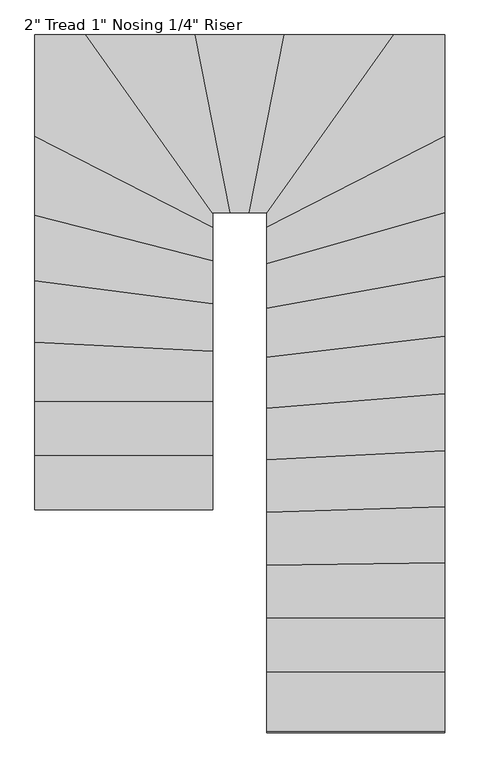
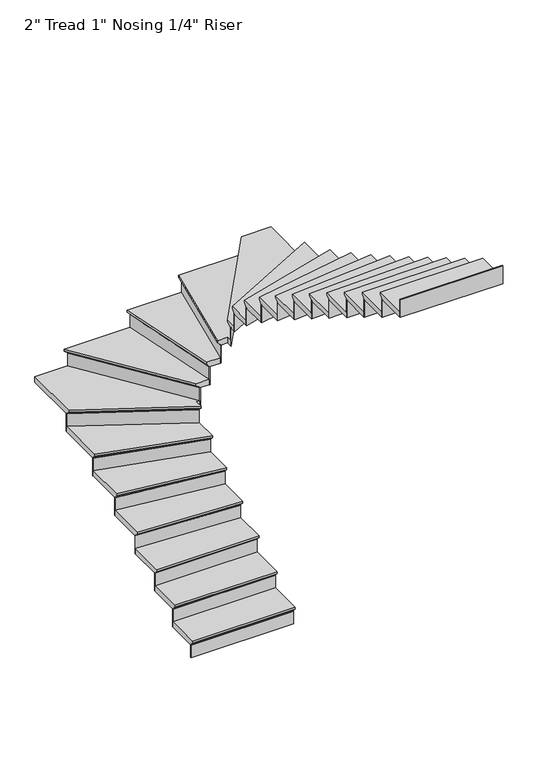
"""IFC4 building model written with IfcOpenShell, lengths in millimetres: stair flight geometry."""

from ifc_helpers import new_model, si_unit, origin, place, context, project, spatial, faceted_brep, source, transform, mapped, element, save


def stair_flight_43e61283(model_context):
    return source(origin(), model_context, "Body", "Brep", [
        faceted_brep([(-6883.2021832, -1637.5895999, 150.2833333), (-6883.2021832, -1637.5895999, 169.3333333), (-7797.6021832, -1637.5895999, 169.3333333), (-7797.6021832, -1637.5895999, 150.2833333), (-6883.2021832, -1612.1895999, 124.8833333), (-7797.6021832, -1612.1895999, 124.8833333), (-6883.2021832, -1332.7895999, 169.3333333), (-7797.6021832, -1332.7895999, 169.3333333), (-7797.6021832, -1612.1895999, 118.5333333), (-7797.6021832, -1332.7895999, 118.5333333), (-6883.2021832, -1332.7895999, 118.5333333), (-6883.2021832, -1612.1895999, 118.5333333)], [[[0, 1, 2, 3]], [[4, 0, 3, 5]], [[2, 1, 6, 7]], [[8, 9, 10, 11]], [[2, 7, 9, 8, 5, 3]], [[8, 11, 4, 5]], [[6, 1, 0, 4, 11, 10]], [[7, 6, 10, 9]]]),
        faceted_brep([(-6883.2021832, -1612.1895999, 118.5333333), (-6883.2021832, -1612.1895999, 0.0), (-6883.2021832, -1605.8395999, 0.0), (-6883.2021832, -1605.8395999, 118.5333333), (-7797.6021832, -1612.1895999, 118.5333333), (-7797.6021832, -1605.8395999, 118.5333333), (-7797.6021832, -1605.8395999, 0.0), (-7797.6021832, -1612.1895999, 0.0)], [[[0, 1, 2, 3]], [[4, 5, 6, 7]], [[1, 0, 4, 7]], [[2, 1, 7, 6]], [[3, 2, 6, 5]], [[0, 3, 5, 4]]]),
        faceted_brep([(-6883.2021832, -1332.7895999, 287.8666667), (-6883.2021832, -1332.7895999, 118.5333333), (-6883.2021832, -1326.4395999, 118.5333333), (-6883.2021832, -1326.4395999, 287.8666667), (-7797.6021832, -1332.7895999, 287.8666667), (-7797.6021832, -1326.4395999, 287.8666667), (-7797.6021832, -1326.4395999, 118.5333333), (-7797.6021832, -1332.7895999, 118.5333333)], [[[0, 1, 2, 3]], [[4, 5, 6, 7]], [[1, 0, 4, 7]], [[2, 1, 7, 6]], [[3, 2, 6, 5]], [[0, 3, 5, 4]]]),
        faceted_brep([(-7797.6021832, -1358.1895999, 338.6666667), (-6883.2021832, -1358.1895999, 338.6666667), (-6883.2021832, -1053.3895999, 338.6666667), (-7797.6021832, -1053.3895999, 338.6666667), (-7797.6021832, -1332.7895999, 287.8666667), (-7797.6021832, -1053.3895999, 287.8666667), (-6883.2021832, -1053.3895999, 287.8666667), (-6883.2021832, -1332.7895999, 287.8666667), (-7797.6021832, -1332.7895999, 294.2166667), (-7797.6021832, -1358.1895999, 319.6166667), (-6883.2021832, -1332.7895999, 294.2166667), (-6883.2021832, -1358.1895999, 319.6166667)], [[[0, 1, 2, 3]], [[4, 5, 6, 7]], [[0, 3, 5, 4, 8, 9]], [[4, 7, 10, 8]], [[2, 1, 11, 10, 7, 6]], [[3, 2, 6, 5]], [[11, 1, 0, 9]], [[10, 11, 9, 8]]]),
        faceted_brep([(-6883.2021832, -1053.3895999, 457.2), (-6883.2021832, -1053.3895999, 287.8666667), (-6883.2021832, -1047.0395999, 287.8666667), (-6883.2021832, -1047.0395999, 457.2), (-7797.6021832, -1053.3895999, 457.2), (-7797.6021832, -1047.0395999, 457.2), (-7797.6021832, -1047.0395999, 287.8666667), (-7797.6021832, -1053.3895999, 287.8666667)], [[[0, 1, 2, 3]], [[4, 5, 6, 7]], [[1, 0, 4, 7]], [[2, 1, 7, 6]], [[3, 2, 6, 5]], [[0, 3, 5, 4]]]),
        faceted_brep([(-7797.6021832, -1078.7895999, 508.0), (-6883.2021832, -1078.7895999, 508.0), (-6883.2021832, -797.7224384, 508.0), (-7797.6021832, -750.188168, 508.0), (-7797.6021832, -1053.3895999, 457.2), (-7797.6021832, -750.188168, 457.2), (-6883.2021832, -797.7224384, 457.2), (-6883.2021832, -1053.3895999, 457.2), (-7797.6021832, -1053.3895999, 463.55), (-7797.6021832, -1078.7895999, 488.95), (-6883.2021832, -1053.3895999, 463.55), (-6883.2021832, -1078.7895999, 488.95)], [[[0, 1, 2, 3]], [[4, 5, 6, 7]], [[0, 3, 5, 4, 8, 9]], [[4, 7, 10, 8]], [[2, 1, 11, 10, 7, 6]], [[3, 2, 6, 5]], [[11, 1, 0, 9]], [[10, 11, 9, 8]]]),
        faceted_brep([(-6883.2021832, -797.7224384, 626.5333333), (-6883.2021832, -797.7224384, 457.2), (-6883.2021832, -791.3638643, 457.2), (-6883.2021832, -791.3638643, 626.5333333), (-7797.6021832, -750.188168, 626.5333333), (-7797.6021832, -743.8295939, 626.5333333), (-7797.6021832, -743.8295939, 457.2), (-7797.6021832, -750.188168, 457.2)], [[[0, 1, 2, 3]], [[4, 5, 6, 7]], [[1, 0, 4, 7]], [[2, 1, 7, 6]], [[3, 2, 6, 5]], [[0, 3, 5, 4]]]),
        faceted_brep([(-7797.6021832, -775.6224647, 677.3333333), (-6883.2021832, -823.1567351, 677.3333333), (-6883.2021832, -553.5557386, 677.3333333), (-7797.6021832, -435.199687, 677.3333333), (-7797.6021832, -750.188168, 626.5333333), (-7797.6021832, -435.199687, 626.5333333), (-6883.2021832, -553.5557386, 626.5333333), (-6883.2021832, -797.7224384, 626.5333333), (-7797.6021832, -750.188168, 632.8833333), (-7797.6021832, -775.6224647, 658.2833333), (-6883.2021832, -797.7224384, 632.8833333), (-6883.2021832, -823.1567351, 658.2833333)], [[[0, 1, 2, 3]], [[4, 5, 6, 7]], [[0, 3, 5, 4, 8, 9]], [[4, 7, 10, 8]], [[2, 1, 11, 10, 7, 6]], [[3, 2, 6, 5]], [[11, 1, 0, 9]], [[10, 11, 9, 8]]]),
        faceted_brep([(-6883.2021832, -553.5557386, 795.8666667), (-6883.2021832, -553.5557386, 626.5333333), (-6883.2021832, -547.1527668, 626.5333333), (-6883.2021832, -547.1527668, 795.8666667), (-7797.6021832, -435.199687, 795.8666667), (-7797.6021832, -428.7967152, 795.8666667), (-7797.6021832, -428.7967152, 626.5333333), (-7797.6021832, -435.199687, 626.5333333)], [[[0, 1, 2, 3]], [[4, 5, 6, 7]], [[1, 0, 4, 7]], [[2, 1, 7, 6]], [[3, 2, 6, 5]], [[0, 3, 5, 4]]]),
        faceted_brep([(-7797.6021832, -460.8115741, 846.6666667), (-6883.2021832, -579.1676257, 846.6666667), (-6883.2021832, -331.9285161, 846.6666667), (-7797.6021832, -96.7980687, 846.6666667), (-7797.6021832, -435.199687, 795.8666667), (-7797.6021832, -96.7980687, 795.8666667), (-6883.2021832, -331.9285161, 795.8666667), (-6883.2021832, -553.5557386, 795.8666667), (-7797.6021832, -435.199687, 802.2166667), (-7797.6021832, -460.8115741, 827.6166667), (-6883.2021832, -553.5557386, 802.2166667), (-6883.2021832, -579.1676257, 827.6166667)], [[[0, 1, 2, 3]], [[4, 5, 6, 7]], [[0, 3, 5, 4, 8, 9]], [[4, 7, 10, 8]], [[2, 1, 11, 10, 7, 6]], [[3, 2, 6, 5]], [[11, 1, 0, 9]], [[10, 11, 9, 8]]]),
        faceted_brep([(-6883.2021832, -331.9285161, 965.2), (-6883.2021832, -331.9285161, 795.8666667), (-6883.2021832, -325.3719393, 795.8666667), (-6883.2021832, -325.3719393, 965.2), (-7797.6021832, -96.7980687, 965.2), (-7797.6021832, -90.2414919, 965.2), (-7797.6021832, -90.2414919, 795.8666667), (-7797.6021832, -96.7980687, 795.8666667)], [[[0, 1, 2, 3]], [[4, 5, 6, 7]], [[1, 0, 4, 7]], [[2, 1, 7, 6]], [[3, 2, 6, 5]], [[0, 3, 5, 4]]]),
        faceted_brep([(-7797.6021832, -123.0243762, 1016.0), (-6883.2021832, -358.1548236, 1016.0), (-6883.2021832, -155.5818801, 1016.0), (-7797.6021832, 313.2427413, 1016.0), (-7797.6021832, -96.7980687, 965.2), (-7797.6021832, 313.2427413, 965.2), (-6883.2021832, -155.5818801, 965.2), (-6883.2021832, -331.9285161, 965.2), (-7797.6021832, -96.7980687, 971.55), (-7797.6021832, -123.0243762, 996.95), (-6883.2021832, -331.9285161, 971.55), (-6883.2021832, -358.1548236, 996.95)], [[[0, 1, 2, 3]], [[4, 5, 6, 7]], [[0, 3, 5, 4, 8, 9]], [[4, 7, 10, 8]], [[2, 1, 11, 10, 7, 6]], [[3, 2, 6, 5]], [[11, 1, 0, 9]], [[10, 11, 9, 8]]]),
        faceted_brep([(-6883.2021832, -155.5818801, 1134.5333333), (-6883.2021832, -155.5818801, 965.2), (-6883.2021832, -148.4458969, 965.2), (-6883.2021832, -148.4458969, 1134.5333333), (-7797.6021832, 313.2427413, 1134.5333333), (-7797.6021832, 320.3787244, 1134.5333333), (-7797.6021832, 320.3787244, 965.2), (-7797.6021832, 313.2427413, 965.2)], [[[0, 1, 2, 3]], [[4, 5, 6, 7]], [[1, 0, 4, 7]], [[2, 1, 7, 6]], [[3, 2, 6, 5]], [[0, 3, 5, 4]]]),
        faceted_brep([(-7503.9210495, 804.542092, 1185.3333333), (-7797.6021832, 804.542092, 1185.3333333), (-7797.6021832, 284.6988087, 1185.3333333), (-6883.2021832, -184.1258126, 1185.3333333), (-6883.2021832, -109.857908, 1185.3333333), (-6853.6471003, -109.857908, 1185.3333333), (-7797.6021832, 804.542092, 1134.5333333), (-7503.9210495, 804.542092, 1134.5333333), (-6853.6471003, -109.857908, 1134.5333333), (-6883.2021832, -109.857908, 1134.5333333), (-6883.2021832, -155.5818801, 1134.5333333), (-7797.6021832, 313.2427413, 1134.5333333), (-7797.6021832, 313.2427413, 1140.8833333), (-7797.6021832, 284.6988087, 1166.2833333), (-6883.2021832, -155.5818801, 1140.8833333), (-6883.2021832, -184.1258126, 1166.2833333)], [[[0, 1, 2, 3, 4, 5]], [[6, 7, 8, 9, 10, 11]], [[1, 0, 7, 6]], [[2, 1, 6, 11, 12, 13]], [[11, 10, 14, 12]], [[4, 3, 15, 14, 10, 9]], [[5, 4, 9, 8]], [[0, 5, 8, 7]], [[15, 3, 2, 13]], [[14, 15, 13, 12]]]),
        faceted_brep([(-6853.6471003, -109.857908, 1303.8666667), (-6853.6471003, -109.857908, 1134.5333333), (-6845.8551255, -109.857908, 1134.5333333), (-6845.8551255, -109.857908, 1303.8666667), (-7503.9210495, 804.542092, 1303.8666667), (-7496.1290747, 804.542092, 1303.8666667), (-7496.1290747, 804.542092, 1134.5333333), (-7503.9210495, 804.542092, 1134.5333333)], [[[0, 1, 2, 3]], [[4, 5, 6, 7]], [[1, 0, 4, 7]], [[2, 1, 7, 6]], [[3, 2, 6, 5]], [[0, 3, 5, 4]]]),
        faceted_brep([(-7535.0889487, 804.542092, 1354.6666667), (-6884.8149995, -109.857908, 1354.6666667), (-6767.1930133, -109.857908, 1354.6666667), (-6947.4338696, 804.542092, 1354.6666667), (-7503.9210495, 804.542092, 1303.8666667), (-6947.4338696, 804.542092, 1303.8666667), (-6767.1930133, -109.857908, 1303.8666667), (-6853.6471003, -109.857908, 1303.8666667), (-7503.9210495, 804.542092, 1310.2166667), (-7535.0889487, 804.542092, 1335.6166667), (-6853.6471003, -109.857908, 1310.2166667), (-6884.8149995, -109.857908, 1335.6166667)], [[[0, 1, 2, 3]], [[4, 5, 6, 7]], [[0, 3, 5, 4, 8, 9]], [[4, 7, 10, 8]], [[2, 1, 11, 10, 7, 6]], [[3, 2, 6, 5]], [[11, 1, 0, 9]], [[10, 11, 9, 8]]]),
        faceted_brep([(-6767.1930133, -109.857908, 1473.2), (-6767.1930133, -109.857908, 1303.8666667), (-6760.7208278, -109.857908, 1303.8666667), (-6760.7208278, -109.857908, 1473.2), (-6947.4338696, 804.542092, 1473.2), (-6940.9616842, 804.542092, 1473.2), (-6940.9616842, 804.542092, 1303.8666667), (-6947.4338696, 804.542092, 1303.8666667)], [[[0, 1, 2, 3]], [[4, 5, 6, 7]], [[1, 0, 4, 7]], [[2, 1, 7, 6]], [[3, 2, 6, 5]], [[0, 3, 5, 4]]]),
        faceted_brep([(-6973.3226113, 804.542092, 1524.0), (-6793.081755, -109.857908, 1524.0), (-6668.0338696, -109.857908, 1524.0), (-6487.7930133, 804.542092, 1524.0), (-6947.4338696, 804.542092, 1473.2), (-6487.7930133, 804.542092, 1473.2), (-6668.0338696, -109.857908, 1473.2), (-6767.1930133, -109.857908, 1473.2), (-6947.4338696, 804.542092, 1479.55), (-6973.3226113, 804.542092, 1504.95), (-6767.1930133, -109.857908, 1479.55), (-6793.081755, -109.857908, 1504.95)], [[[0, 1, 2, 3]], [[4, 5, 6, 7]], [[0, 3, 5, 4, 8, 9]], [[4, 7, 10, 8]], [[2, 1, 11, 10, 7, 6]], [[3, 2, 6, 5]], [[11, 1, 0, 9]], [[10, 11, 9, 8]]]),
        faceted_brep([(-6668.0338696, -109.857908, 1642.5333333), (-6668.0338696, -109.857908, 1473.2), (-6661.5616842, -109.857908, 1473.2), (-6661.5616842, -109.857908, 1642.5333333), (-6487.7930133, 804.542092, 1642.5333333), (-6481.3208278, 804.542092, 1642.5333333), (-6481.3208278, 804.542092, 1473.2), (-6487.7930133, 804.542092, 1473.2)], [[[0, 1, 2, 3]], [[4, 5, 6, 7]], [[1, 0, 4, 7]], [[2, 1, 7, 6]], [[3, 2, 6, 5]], [[0, 3, 5, 4]]]),
        faceted_brep([(-6513.681755, 804.542092, 1693.3333333), (-6693.9226113, -109.857908, 1693.3333333), (-6603.8021832, -109.857908, 1693.3333333), (-6603.8021832, -155.9533826, 1693.3333333), (-5920.7475185, 804.542092, 1693.3333333), (-6487.7930133, 804.542092, 1642.5333333), (-5920.7475185, 804.542092, 1642.5333333), (-6603.8021832, -155.9533826, 1642.5333333), (-6603.8021832, -109.857908, 1642.5333333), (-6668.0338696, -109.857908, 1642.5333333), (-6487.7930133, 804.542092, 1648.8833333), (-6513.681755, 804.542092, 1674.2833333), (-6668.0338696, -109.857908, 1648.8833333), (-6693.9226113, -109.857908, 1674.2833333)], [[[0, 1, 2, 3, 4]], [[5, 6, 7, 8, 9]], [[0, 4, 6, 5, 10, 11]], [[5, 9, 12, 10]], [[2, 1, 13, 12, 9, 8]], [[3, 2, 8, 7]], [[4, 3, 7, 6]], [[13, 1, 0, 11]], [[12, 13, 11, 10]]]),
        faceted_brep([(-6603.8021832, -155.9533826, 1811.8666667), (-6603.8021832, -155.9533826, 1642.5333333), (-6603.8021832, -166.9102751, 1642.5333333), (-6603.8021832, -166.9102751, 1811.8666667), (-5920.7475185, 804.542092, 1811.8666667), (-5912.9555437, 804.542092, 1811.8666667), (-5912.9555437, 804.542092, 1642.5333333), (-5920.7475185, 804.542092, 1642.5333333)], [[[0, 1, 2, 3]], [[4, 5, 6, 7]], [[1, 0, 4, 7]], [[2, 1, 7, 6]], [[3, 2, 6, 5]], [[0, 3, 5, 4]]]),
        faceted_brep([(-5689.4021832, 256.1548762, 1862.6666667), (-5689.4021832, 804.542092, 1862.6666667), (-5951.9154177, 804.542092, 1862.6666667), (-6603.8021832, -112.1258126, 1862.6666667), (-6603.8021832, -212.6697451, 1862.6666667), (-5689.4021832, 804.542092, 1811.8666667), (-5689.4021832, 256.1548762, 1811.8666667), (-6603.8021832, -212.6697451, 1811.8666667), (-6603.8021832, -155.9533826, 1811.8666667), (-5920.7475185, 804.542092, 1811.8666667), (-5920.7475185, 804.542092, 1818.2166667), (-5951.9154177, 804.542092, 1843.6166667), (-6603.8021832, -155.9533826, 1818.2166667), (-6603.8021832, -112.1258126, 1843.6166667)], [[[0, 1, 2, 3, 4]], [[5, 6, 7, 8, 9]], [[1, 0, 6, 5]], [[2, 1, 5, 9, 10, 11]], [[9, 8, 12, 10]], [[4, 3, 13, 12, 8, 7]], [[0, 4, 7, 6]], [[13, 3, 2, 11]], [[12, 13, 11, 10]]]),
        faceted_brep([(-6603.8021832, -212.6697451, 1981.2), (-6603.8021832, -212.6697451, 1811.8666667), (-6603.8021832, -219.8057283, 1811.8666667), (-6603.8021832, -219.8057283, 1981.2), (-5689.4021832, 256.1548762, 1981.2), (-5689.4021832, 249.0188931, 1981.2), (-5689.4021832, 249.0188931, 1811.8666667), (-5689.4021832, 256.1548762, 1811.8666667)], [[[0, 1, 2, 3]], [[4, 5, 6, 7]], [[1, 0, 4, 7]], [[2, 1, 7, 6]], [[3, 2, 6, 5]], [[0, 3, 5, 4]]]),
        faceted_brep([(-5689.4021832, 284.6988087, 2032.0), (-6603.8021832, -184.1258126, 2032.0), (-6603.8021832, -398.0396416, 2032.0), (-5689.4021832, -135.9845514, 2032.0), (-5689.4021832, 256.1548762, 1981.2), (-5689.4021832, -135.9845514, 1981.2), (-6603.8021832, -398.0396416, 1981.2), (-6603.8021832, -212.6697451, 1981.2), (-5689.4021832, 256.1548762, 1987.55), (-5689.4021832, 284.6988087, 2012.95), (-6603.8021832, -212.6697451, 1987.55), (-6603.8021832, -184.1258126, 2012.95)], [[[0, 1, 2, 3]], [[4, 5, 6, 7]], [[0, 3, 5, 4, 8, 9]], [[4, 7, 10, 8]], [[2, 1, 11, 10, 7, 6]], [[3, 2, 6, 5]], [[11, 1, 0, 9]], [[10, 11, 9, 8]]]),
        faceted_brep([(-6603.8021832, -398.0396416, 2150.5333333), (-6603.8021832, -398.0396416, 1981.2), (-6603.8021832, -404.6452657, 1981.2), (-6603.8021832, -404.6452657, 2150.5333333), (-5689.4021832, -135.9845514, 2150.5333333), (-5689.4021832, -142.5901756, 2150.5333333), (-5689.4021832, -142.5901756, 1981.2), (-5689.4021832, -135.9845514, 1981.2)], [[[0, 1, 2, 3]], [[4, 5, 6, 7]], [[1, 0, 4, 7]], [[2, 1, 7, 6]], [[3, 2, 6, 5]], [[0, 3, 5, 4]]]),
        faceted_brep([(-5689.4021832, -109.5620548, 2201.3333333), (-6603.8021832, -371.617145, 2201.3333333), (-6603.8021832, -628.5095566, 2201.3333333), (-5689.4021832, -463.0941664, 2201.3333333), (-5689.4021832, -135.9845514, 2150.5333333), (-5689.4021832, -463.0941664, 2150.5333333), (-6603.8021832, -628.5095566, 2150.5333333), (-6603.8021832, -398.0396416, 2150.5333333), (-5689.4021832, -135.9845514, 2156.8833333), (-5689.4021832, -109.5620548, 2182.2833333), (-6603.8021832, -398.0396416, 2156.8833333), (-6603.8021832, -371.617145, 2182.2833333)], [[[0, 1, 2, 3]], [[4, 5, 6, 7]], [[0, 3, 5, 4, 8, 9]], [[4, 7, 10, 8]], [[2, 1, 11, 10, 7, 6]], [[3, 2, 6, 5]], [[11, 1, 0, 9]], [[10, 11, 9, 8]]]),
        faceted_brep([(-6603.8021832, -628.5095566, 2319.8666667), (-6603.8021832, -628.5095566, 2150.5333333), (-6603.8021832, -634.962622, 2150.5333333), (-6603.8021832, -634.962622, 2319.8666667), (-5689.4021832, -463.0941664, 2319.8666667), (-5689.4021832, -469.5472318, 2319.8666667), (-5689.4021832, -469.5472318, 2150.5333333), (-5689.4021832, -463.0941664, 2150.5333333)], [[[0, 1, 2, 3]], [[4, 5, 6, 7]], [[1, 0, 4, 7]], [[2, 1, 7, 6]], [[3, 2, 6, 5]], [[0, 3, 5, 4]]]),
        faceted_brep([(-5689.4021832, -437.2819048, 2370.6666667), (-6603.8021832, -602.697295, 2370.6666667), (-6603.8021832, -879.5159372, 2370.6666667), (-5689.4021832, -770.4235202, 2370.6666667), (-5689.4021832, -463.0941664, 2319.8666667), (-5689.4021832, -770.4235202, 2319.8666667), (-6603.8021832, -879.5159372, 2319.8666667), (-6603.8021832, -628.5095566, 2319.8666667), (-5689.4021832, -463.0941664, 2326.2166667), (-5689.4021832, -437.2819048, 2351.6166667), (-6603.8021832, -628.5095566, 2326.2166667), (-6603.8021832, -602.697295, 2351.6166667)], [[[0, 1, 2, 3]], [[4, 5, 6, 7]], [[0, 3, 5, 4, 8, 9]], [[4, 7, 10, 8]], [[2, 1, 11, 10, 7, 6]], [[3, 2, 6, 5]], [[11, 1, 0, 9]], [[10, 11, 9, 8]]]),
        faceted_brep([(-6603.8021832, -879.5159372, 2489.2), (-6603.8021832, -879.5159372, 2319.8666667), (-6603.8021832, -885.9109694, 2319.8666667), (-6603.8021832, -885.9109694, 2489.2), (-5689.4021832, -770.4235202, 2489.2), (-5689.4021832, -776.8185524, 2489.2), (-5689.4021832, -776.8185524, 2319.8666667), (-5689.4021832, -770.4235202, 2319.8666667)], [[[0, 1, 2, 3]], [[4, 5, 6, 7]], [[1, 0, 4, 7]], [[2, 1, 7, 6]], [[3, 2, 6, 5]], [[0, 3, 5, 4]]]),
        faceted_brep([(-5689.4021832, -744.8433914, 2540.0), (-6603.8021832, -853.9358084, 2540.0), (-6603.8021832, -1140.3742729, 2540.0), (-5689.4021832, -1068.1630862, 2540.0), (-5689.4021832, -770.4235202, 2489.2), (-5689.4021832, -1068.1630862, 2489.2), (-6603.8021832, -1140.3742729, 2489.2), (-6603.8021832, -879.5159372, 2489.2), (-5689.4021832, -770.4235202, 2495.55), (-5689.4021832, -744.8433914, 2520.95), (-6603.8021832, -879.5159372, 2495.55), (-6603.8021832, -853.9358084, 2520.95)], [[[0, 1, 2, 3]], [[4, 5, 6, 7]], [[0, 3, 5, 4, 8, 9]], [[4, 7, 10, 8]], [[2, 1, 11, 10, 7, 6]], [[3, 2, 6, 5]], [[11, 1, 0, 9]], [[10, 11, 9, 8]]]),
        faceted_brep([(-6603.8021832, -1140.3742729, 2658.5333333), (-6603.8021832, -1140.3742729, 2489.2), (-6603.8021832, -1146.7440428, 2489.2), (-6603.8021832, -1146.7440428, 2658.5333333), (-5689.4021832, -1068.1630862, 2658.5333333), (-5689.4021832, -1074.5328561, 2658.5333333), (-5689.4021832, -1074.5328561, 2489.2), (-5689.4021832, -1068.1630862, 2489.2)], [[[0, 1, 2, 3]], [[4, 5, 6, 7]], [[1, 0, 4, 7]], [[2, 1, 7, 6]], [[3, 2, 6, 5]], [[0, 3, 5, 4]]]),
        faceted_brep([(-5689.4021832, -1042.6840066, 2709.3333333), (-6603.8021832, -1114.8951932, 2709.3333333), (-6603.8021832, -1406.7154394, 2709.3333333), (-5689.4021832, -1360.5285227, 2709.3333333), (-5689.4021832, -1068.1630862, 2658.5333333), (-5689.4021832, -1360.5285227, 2658.5333333), (-6603.8021832, -1406.7154394, 2658.5333333), (-6603.8021832, -1140.3742729, 2658.5333333), (-5689.4021832, -1068.1630862, 2664.8833333), (-5689.4021832, -1042.6840066, 2690.2833333), (-6603.8021832, -1140.3742729, 2664.8833333), (-6603.8021832, -1114.8951932, 2690.2833333)], [[[0, 1, 2, 3]], [[4, 5, 6, 7]], [[0, 3, 5, 4, 8, 9]], [[4, 7, 10, 8]], [[2, 1, 11, 10, 7, 6]], [[3, 2, 6, 5]], [[11, 1, 0, 9]], [[10, 11, 9, 8]]]),
        faceted_brep([(-6603.8021832, -1406.7154394, 2827.8666667), (-6603.8021832, -1406.7154394, 2658.5333333), (-6603.8021832, -1413.0735347, 2658.5333333), (-6603.8021832, -1413.0735347, 2827.8666667), (-5689.4021832, -1360.5285227, 2827.8666667), (-5689.4021832, -1366.886618, 2827.8666667), (-5689.4021832, -1366.886618, 2658.5333333), (-5689.4021832, -1360.5285227, 2658.5333333)], [[[0, 1, 2, 3]], [[4, 5, 6, 7]], [[1, 0, 4, 7]], [[2, 1, 7, 6]], [[3, 2, 6, 5]], [[0, 3, 5, 4]]]),
        faceted_brep([(-5689.4021832, -1335.0961416, 2878.6666667), (-6603.8021832, -1381.2830582, 2878.6666667), (-6603.8021832, -1676.420866, 2878.6666667), (-5689.4021832, -1649.5802142, 2878.6666667), (-5689.4021832, -1360.5285227, 2827.8666667), (-5689.4021832, -1649.5802142, 2827.8666667), (-6603.8021832, -1676.420866, 2827.8666667), (-6603.8021832, -1406.7154394, 2827.8666667), (-5689.4021832, -1360.5285227, 2834.2166667), (-5689.4021832, -1335.0961416, 2859.6166667), (-6603.8021832, -1406.7154394, 2834.2166667), (-6603.8021832, -1381.2830582, 2859.6166667)], [[[0, 1, 2, 3]], [[4, 5, 6, 7]], [[0, 3, 5, 4, 8, 9]], [[4, 7, 10, 8]], [[2, 1, 11, 10, 7, 6]], [[3, 2, 6, 5]], [[11, 1, 0, 9]], [[10, 11, 9, 8]]]),
        faceted_brep([(-6603.8021832, -1676.420866, 2997.2), (-6603.8021832, -1676.420866, 2827.8666667), (-6603.8021832, -1682.773601, 2827.8666667), (-6603.8021832, -1682.773601, 2997.2), (-5689.4021832, -1649.5802142, 2997.2), (-5689.4021832, -1655.9329492, 2997.2), (-5689.4021832, -1655.9329492, 2827.8666667), (-5689.4021832, -1649.5802142, 2827.8666667)], [[[0, 1, 2, 3]], [[4, 5, 6, 7]], [[1, 0, 4, 7]], [[2, 1, 7, 6]], [[3, 2, 6, 5]], [[0, 3, 5, 4]]]),
        faceted_brep([(-5689.4021832, -1624.169274, 3048.0), (-6603.8021832, -1651.0099258, 3048.0), (-6603.8021832, -1948.338875, 3048.0), (-5689.4021832, -1936.4446223, 3048.0), (-5689.4021832, -1649.5802142, 2997.2), (-5689.4021832, -1936.4446223, 2997.2), (-6603.8021832, -1948.338875, 2997.2), (-6603.8021832, -1676.420866, 2997.2), (-5689.4021832, -1649.5802142, 3003.55), (-5689.4021832, -1624.169274, 3028.95), (-6603.8021832, -1676.420866, 3003.55), (-6603.8021832, -1651.0099258, 3028.95)], [[[0, 1, 2, 3]], [[4, 5, 6, 7]], [[0, 3, 5, 4, 8, 9]], [[4, 7, 10, 8]], [[2, 1, 11, 10, 7, 6]], [[3, 2, 6, 5]], [[11, 1, 0, 9]], [[10, 11, 9, 8]]]),
        faceted_brep([(-6603.8021832, -1948.338875, 3166.5333333), (-6603.8021832, -1948.338875, 2997.2), (-6603.8021832, -1954.6894122, 2997.2), (-6603.8021832, -1954.6894122, 3166.5333333), (-5689.4021832, -1936.4446223, 3166.5333333), (-5689.4021832, -1942.7951595, 3166.5333333), (-5689.4021832, -1942.7951595, 2997.2), (-5689.4021832, -1936.4446223, 2997.2)], [[[0, 1, 2, 3]], [[4, 5, 6, 7]], [[1, 0, 4, 7]], [[2, 1, 7, 6]], [[3, 2, 6, 5]], [[0, 3, 5, 4]]]),
        faceted_brep([(-5689.4021832, -1911.0424735, 3217.3333333), (-6603.8021832, -1922.9367263, 3217.3333333), (-6603.8021832, -2221.7895999, 3217.3333333), (-5689.4021832, -2221.7895999, 3217.3333333), (-5689.4021832, -1936.4446223, 3166.5333333), (-5689.4021832, -2221.7895999, 3166.5333333), (-6603.8021832, -2221.7895999, 3166.5333333), (-6603.8021832, -1948.338875, 3166.5333333), (-5689.4021832, -1936.4446223, 3172.8833333), (-5689.4021832, -1911.0424735, 3198.2833333), (-6603.8021832, -1948.338875, 3172.8833333), (-6603.8021832, -1922.9367263, 3198.2833333)], [[[0, 1, 2, 3]], [[4, 5, 6, 7]], [[0, 3, 5, 4, 8, 9]], [[4, 7, 10, 8]], [[2, 1, 11, 10, 7, 6]], [[3, 2, 6, 5]], [[11, 1, 0, 9]], [[10, 11, 9, 8]]]),
        faceted_brep([(-6603.8021832, -2221.7895999, 3335.8666667), (-6603.8021832, -2221.7895999, 3166.5333333), (-6603.8021832, -2228.1395999, 3166.5333333), (-6603.8021832, -2228.1395999, 3335.8666667), (-5689.4021832, -2221.7895999, 3335.8666667), (-5689.4021832, -2228.1395999, 3335.8666667), (-5689.4021832, -2228.1395999, 3166.5333333), (-5689.4021832, -2221.7895999, 3166.5333333)], [[[0, 1, 2, 3]], [[4, 5, 6, 7]], [[1, 0, 4, 7]], [[2, 1, 7, 6]], [[3, 2, 6, 5]], [[0, 3, 5, 4]]]),
        faceted_brep([(-5689.4021832, -2196.3895999, 3386.6666667), (-6603.8021832, -2196.3895999, 3386.6666667), (-6603.8021832, -2501.1895999, 3386.6666667), (-5689.4021832, -2501.1895999, 3386.6666667), (-5689.4021832, -2221.7895999, 3335.8666667), (-5689.4021832, -2501.1895999, 3335.8666667), (-6603.8021832, -2501.1895999, 3335.8666667), (-6603.8021832, -2221.7895999, 3335.8666667), (-5689.4021832, -2221.7895999, 3342.2166667), (-5689.4021832, -2196.3895999, 3367.6166667), (-6603.8021832, -2221.7895999, 3342.2166667), (-6603.8021832, -2196.3895999, 3367.6166667)], [[[0, 1, 2, 3]], [[4, 5, 6, 7]], [[0, 3, 5, 4, 8, 9]], [[4, 7, 10, 8]], [[2, 1, 11, 10, 7, 6]], [[3, 2, 6, 5]], [[11, 1, 0, 9]], [[10, 11, 9, 8]]]),
        faceted_brep([(-6603.8021832, -2501.1895999, 3505.2), (-6603.8021832, -2501.1895999, 3335.8666667), (-6603.8021832, -2507.5395999, 3335.8666667), (-6603.8021832, -2507.5395999, 3505.2), (-5689.4021832, -2501.1895999, 3505.2), (-5689.4021832, -2507.5395999, 3505.2), (-5689.4021832, -2507.5395999, 3335.8666667), (-5689.4021832, -2501.1895999, 3335.8666667)], [[[0, 1, 2, 3]], [[4, 5, 6, 7]], [[1, 0, 4, 7]], [[2, 1, 7, 6]], [[3, 2, 6, 5]], [[0, 3, 5, 4]]]),
        faceted_brep([(-6603.8021832, -2780.5895999, 3674.5333333), (-6603.8021832, -2780.5895999, 3505.2), (-6603.8021832, -2786.9395999, 3505.2), (-6603.8021832, -2786.9395999, 3674.5333333), (-5689.4021832, -2780.5895999, 3674.5333333), (-5689.4021832, -2786.9395999, 3674.5333333), (-5689.4021832, -2786.9395999, 3505.2), (-5689.4021832, -2780.5895999, 3505.2)], [[[0, 1, 2, 3]], [[4, 5, 6, 7]], [[1, 0, 4, 7]], [[2, 1, 7, 6]], [[3, 2, 6, 5]], [[0, 3, 5, 4]]]),
        faceted_brep([(-5689.4021832, -2475.7895999, 3556.0), (-6603.8021832, -2475.7895999, 3556.0), (-6603.8021832, -2780.5895999, 3556.0), (-5689.4021832, -2780.5895999, 3556.0), (-5689.4021832, -2501.1895999, 3505.2), (-5689.4021832, -2780.5895999, 3505.2), (-6603.8021832, -2780.5895999, 3505.2), (-6603.8021832, -2501.1895999, 3505.2), (-5689.4021832, -2501.1895999, 3511.55), (-5689.4021832, -2475.7895999, 3536.95), (-6603.8021832, -2501.1895999, 3511.55), (-6603.8021832, -2475.7895999, 3536.95)], [[[0, 1, 2, 3]], [[4, 5, 6, 7]], [[0, 3, 5, 4, 8, 9]], [[4, 7, 10, 8]], [[2, 1, 11, 10, 7, 6]], [[3, 2, 6, 5]], [[11, 1, 0, 9]], [[10, 11, 9, 8]]]),
    ])


if __name__ == "__main__":
    model = new_model("IFC4")
    model_context = context("Model", 3, world=origin())
    ifc_project = project(units=[si_unit("LENGTHUNIT", "METRE", prefix="MILLI")], contexts=[model_context])
    site = spatial("IfcSite", under=ifc_project)
    building = spatial("IfcBuilding", under=site)
    placement = place(None, origin())
    stair_flight_shape = stair_flight_43e61283(model_context)
    element("IfcStairFlight", 1, ObjectType="2\" Tread 1\" Nosing 1/4\" Riser", at=placement, inside=building, context=model_context, shape_type="MappedRepresentation", body=[
        mapped(stair_flight_shape, transform((0.0, 0.0, 0.0), x_axis=(1.0, 0.0, 0.0), y_axis=(0.0, 1.0, 0.0), z_axis=(0.0, 0.0, 1.0))),
    ])
    save(model, "model.ifc")
